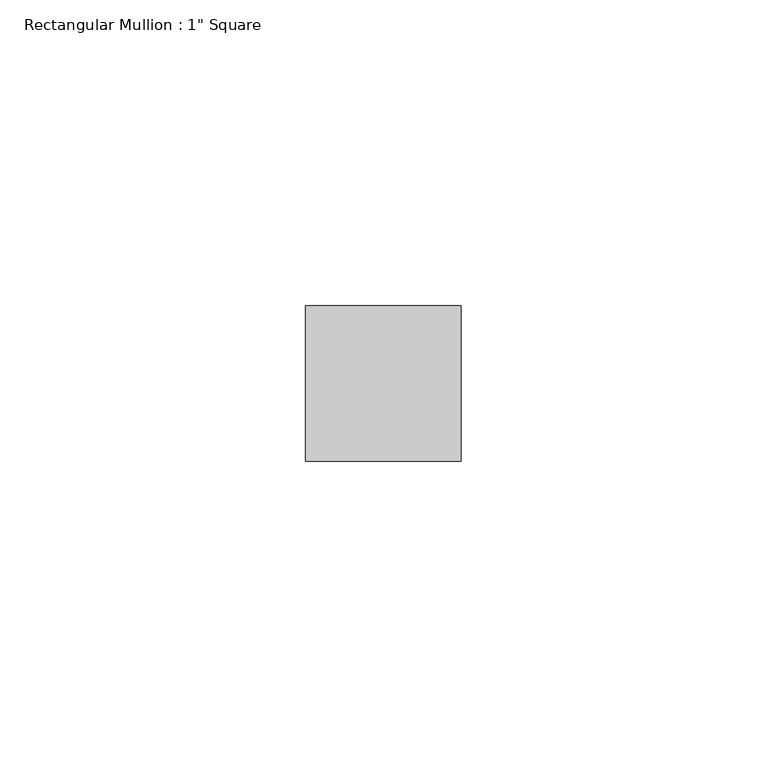
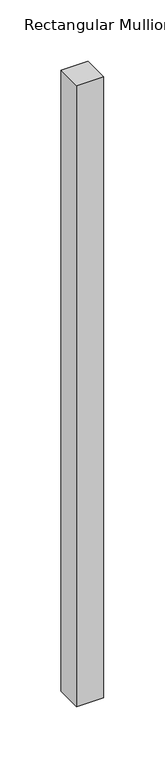
"""IFC4 building model written with IfcOpenShell, lengths in millimetres: member geometry."""

from ifc_helpers import new_model, si_unit, frame, origin, place, context, project, spatial, polyline, outline, extrude, source, transform, mapped, element, save


def member_910a056f(model_context):
    return source(origin(), model_context, "Body", "SweptSolid", [
        extrude(outline(polyline([(12.7, 12.7), (12.7, -12.7), (-12.7, -12.7), (-12.7, 12.7), (12.7, 12.7)])), frame((0.0, 0.0, -618.0666667), z_axis=(0.0, 0.0, 1.0), x_axis=(1.0, 0.0, 0.0)), (0.0, 0.0, 1.0), 618.0666667),
    ])


if __name__ == "__main__":
    model = new_model("IFC4")
    model_context = context("Model", 3, world=origin())
    ifc_project = project(units=[si_unit("LENGTHUNIT", "METRE", prefix="MILLI")], contexts=[model_context])
    site = spatial("IfcSite", under=ifc_project)
    building = spatial("IfcBuilding", under=site)
    placement = place(None, origin())
    member_shape = member_910a056f(model_context)
    element("IfcMember", 1, ObjectType="Rectangular Mullion : 1\" Square", at=placement, inside=building, context=model_context, shape_type="MappedRepresentation", body=[
        mapped(member_shape, transform((0.0, 0.0, 0.0), x_axis=(1.0, 0.0, 0.0), y_axis=(0.0, 1.0, 0.0), z_axis=(0.0, 0.0, 1.0))),
    ])
    save(model, "model.ifc")

# Revit data of these elements
# Type "Rectangular Mullion : 1\" Square"
#   built-in parameter 1007304 = 0.0833333 (stored number, unit not read)
#   built-in parameter 1007301 = 0.0416667 (stored number, unit not read)
#   built-in parameter 1007300 = 0.0416667 (stored number, unit not read)
# Element 1 (IfcMember, "Rectangular Mullion : 1\" Square")
#   Materials on its faces: "Aluminum"
# Materials
#   "Aluminum": class "Metal", colour RGB 247 247 247, transparency 0, Description = "Aluminum 6061", Cost = 0
